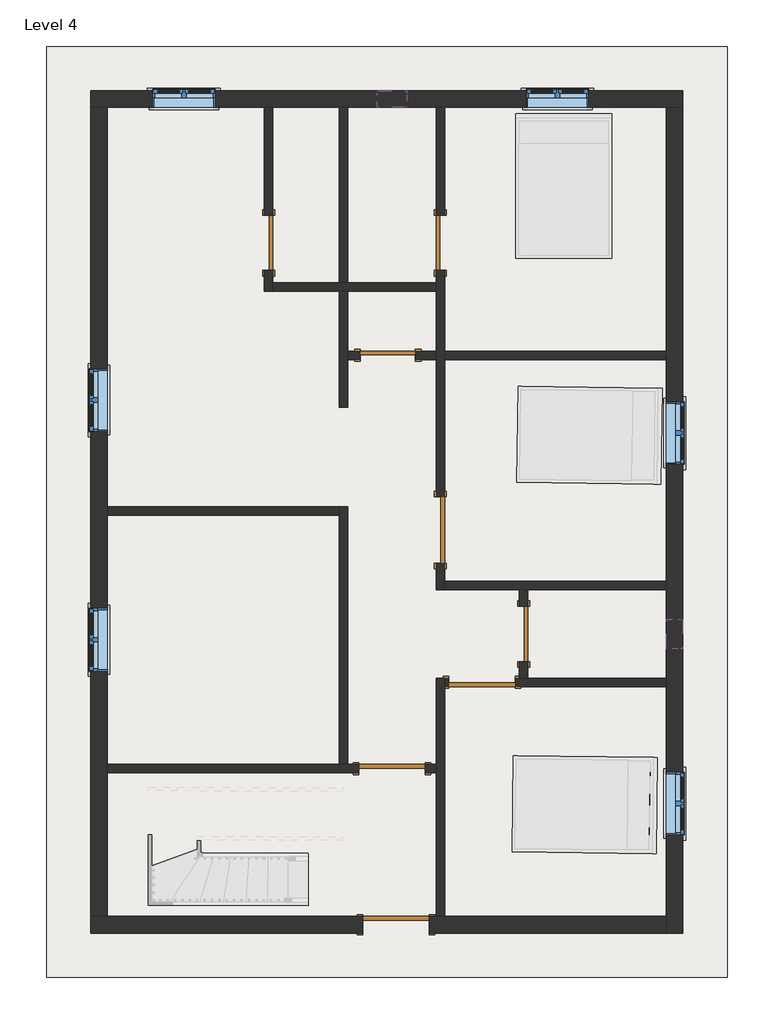
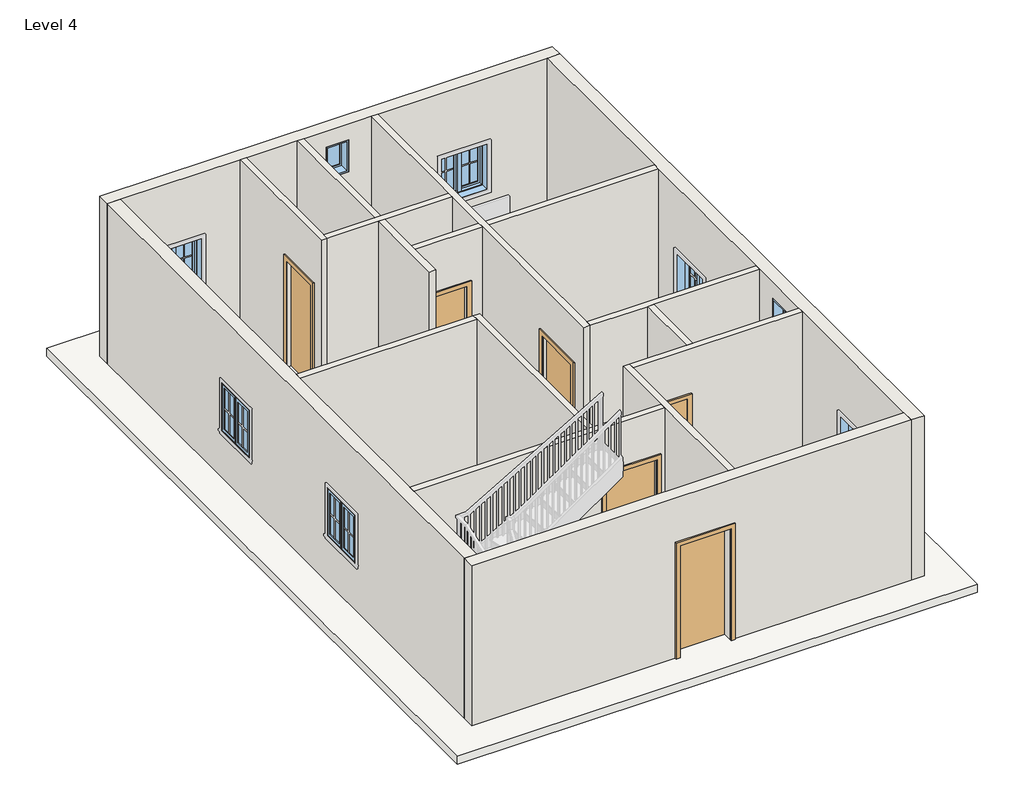
# One storey, part 1 of 3: 17 walls, 8 doors, 8 windows, 1 roof.
"""IFC4 building model written with IfcOpenShell, lengths in millimetres."""

from ifc_helpers import new_model, si_unit, frame, origin, place, context, project, spatial, polyline, outline, extrude, faceted_brep, transform, mapped, element, save
from components import door_d8f5dbb5, door_f2b275c1, door_e5f9f3c4, door_305aa2a5, door_0ca8825f, window_aa618e30, window_339605e1

model = new_model("IFC4")

# Units and contexts
model_context = context("Model", 3, world=origin())
ifc_project = project(units=[si_unit("LENGTHUNIT", "METRE", prefix="MILLI")], contexts=[model_context])

# Site, building, storey
site = spatial("IfcSite", under=ifc_project)
building = spatial("IfcBuilding", under=site)
storey = spatial("IfcBuildingStorey", under=building, Name="Level 4", Elevation=6400.8)

# Doors
placement = place(None, origin())
door_shape = door_d8f5dbb5(model_context)
element("IfcDoor", 1, ObjectType="Single-Flush : 30\" x 80\"", at=placement, inside=storey, context=model_context, shape_type="MappedRepresentation", body=[
    mapped(door_shape, transform((-2883.8867314, 4242.0321212, 6400.8), x_axis=(0.0, -1.0, 0.0), y_axis=(1.0, 0.0, 0.0), z_axis=(0.0, 0.0, 1.0))),
])
door_2_shape = door_f2b275c1(model_context)
element("IfcDoor", 2, ObjectType="Single-Flush : 30\" x 80\"", at=placement, inside=storey, context=model_context, shape_type="MappedRepresentation", body=[
    mapped(door_2_shape, transform((-521.6867314, 4242.0321212, 6400.8), x_axis=(0.0, -1.0, 0.0), y_axis=(1.0, 0.0, 0.0), z_axis=(0.0, 0.0, 1.0))),
])
element("IfcDoor", 3, ObjectType="Single-Flush : 30\" x 80\"", at=placement, inside=storey, context=model_context, shape_type="MappedRepresentation", body=[
    mapped(door_2_shape, transform((-1245.5867314, 2692.6321212, 6400.8), x_axis=(-1.0, 0.0, 0.0), y_axis=(0.0, -1.0, 0.0), z_axis=(0.0, 0.0, 1.0))),
])
element("IfcDoor", 4, ObjectType="Single-Flush : 30\" x 80\"", at=placement, inside=storey, context=model_context, shape_type="MappedRepresentation", body=[
    mapped(door_2_shape, transform((621.3132686, -1136.4178788, 6400.8), x_axis=(0.0, 1.0, 0.0), y_axis=(-1.0, 0.0, 0.0), z_axis=(0.0, 0.0, 1.0))),
])
door_3_shape = door_e5f9f3c4(model_context)
element("IfcDoor", 5, ObjectType="Single-Flush : 36\" x 84\"", at=placement, inside=storey, context=model_context, shape_type="MappedRepresentation", body=[
    mapped(door_3_shape, transform((-521.6867314, 292.3321212, 6400.8), x_axis=(0.0, -1.0, 0.0), y_axis=(1.0, 0.0, 0.0), z_axis=(0.0, 0.0, 1.0))),
])
element("IfcDoor", 6, ObjectType="Single-Flush : 36\" x 84\"", at=placement, inside=storey, context=model_context, shape_type="MappedRepresentation", body=[
    mapped(door_3_shape, transform((-1188.4367314, -2989.1542682, 6400.8), x_axis=(1.0, 0.0, 0.0), y_axis=(0.0, 1.0, 0.0), z_axis=(0.0, 0.0, 1.0))),
])
door_4_shape = door_305aa2a5(model_context)
element("IfcDoor", 7, ObjectType="Single-Flush : 36\" x 84\"", at=placement, inside=storey, context=model_context, shape_type="MappedRepresentation", body=[
    mapped(door_4_shape, transform((49.8132686, -1803.1678788, 6400.8), x_axis=(1.0, 0.0, 0.0), y_axis=(0.0, 1.0, 0.0), z_axis=(0.0, 0.0, 1.0))),
])
door_5_shape = door_0ca8825f(model_context)
element("IfcDoor", 8, ObjectType="Single-Flush : 36\" x 84\"", at=placement, inside=storey, context=model_context, shape_type="MappedRepresentation", body=[
    mapped(door_5_shape, transform((-1131.2867314, -5136.9178788, 6400.8), x_axis=(1.0, 0.0, 0.0), y_axis=(0.0, 1.0, 0.0), z_axis=(0.0, 0.0, 1.0))),
])

# Roof
element("IfcRoof", 9, ObjectType="Generic - 12\"", at=placement, inside=storey, context=model_context, shape_type="SweptSolid", body=[
    extrude(outline(polyline([(-5938.2367314, 6940.7821212), (3421.6632686, 6940.7821212), (3421.6632686, -5860.8178788), (-5938.2367314, -5860.8178788), (-5938.2367314, 6940.7821212)])), frame((0.0, 0.0, 6248.4), z_axis=(0.0, 0.0, 1.0), x_axis=(1.0, 0.0, 0.0)), (0.0, 0.0, 1.0), 152.4),
])

# Walls
element("IfcWall", 10, ObjectType="wall4.5\"", at=placement, inside=storey, context=model_context, shape_type="Brep", body=[
    faceted_brep([(-2941.0367314, 3861.0321212, 8432.8), (-2941.0367314, 3861.0321212, 6400.8), (-2941.0367314, 3575.2821212, 6400.8), (-2941.0367314, 3575.2821212, 9448.8), (-2941.0367314, 6102.5821212, 9448.8), (-2941.0367314, 6102.5821212, 6400.8), (-2941.0367314, 4623.0321212, 6400.8), (-2941.0367314, 4623.0321212, 8432.8), (-2826.7367314, 3575.2821212, 6400.8), (-2826.7367314, 3689.5821212, 6400.8), (-2826.7367314, 3861.0321212, 6400.8), (-2826.7367314, 3861.0321212, 8432.8), (-2826.7367314, 4623.0321212, 8432.8), (-2826.7367314, 4623.0321212, 6400.8), (-2826.7367314, 6102.5821212, 6400.8), (-2826.7367314, 6102.5821212, 9448.8), (-2826.7367314, 3689.5821212, 9448.8), (-2826.7367314, 3575.2821212, 9448.8)], [[[0, 1, 2, 3, 4, 5, 6, 7]], [[8, 9, 10, 11, 12, 13, 14, 15, 16, 17]], [[6, 5, 14, 13]], [[2, 1, 10, 9, 8]], [[5, 4, 15, 14]], [[3, 2, 8, 17]], [[11, 10, 1, 0]], [[12, 11, 0, 7]], [[13, 12, 7, 6]], [[4, 3, 17, 16, 15]]]),
])
element("IfcWall", 11, ObjectType="wall4.5\"", at=placement, inside=storey, context=model_context, shape_type="Brep", body=[
    faceted_brep([(-2826.7367314, 3575.2821212, 6400.8), (-1912.3367314, 3575.2821212, 6400.8), (-1798.0367314, 3575.2821212, 6400.8), (-578.8367314, 3575.2821212, 6400.8), (-578.8367314, 3575.2821212, 9448.8), (-1798.0367314, 3575.2821212, 9448.8), (-1912.3367314, 3575.2821212, 9448.8), (-2826.7367314, 3575.2821212, 9448.8), (-2826.7367314, 3689.5821212, 6400.8), (-2826.7367314, 3689.5821212, 9448.8), (-1912.3367314, 3689.5821212, 9448.8), (-1798.0367314, 3689.5821212, 9448.8), (-578.8367314, 3689.5821212, 9448.8), (-578.8367314, 3689.5821212, 6400.8), (-1798.0367314, 3689.5821212, 6400.8), (-1912.3367314, 3689.5821212, 6400.8)], [[[0, 1, 2, 3, 4, 5, 6, 7]], [[8, 9, 10, 11, 12, 13, 14, 15]], [[3, 2, 1, 0, 8, 15, 14, 13]], [[0, 7, 9, 8]], [[4, 3, 13, 12]], [[7, 6, 5, 4, 12, 11, 10, 9]]]),
])
element("IfcWall", 12, ObjectType="wall4.5\"", at=placement, inside=storey, context=model_context, shape_type="SweptSolid", body=[
    extrude(outline(polyline([(-1912.3367314, 3689.5821212), (-1912.3367314, 6102.5821212), (-1798.0367314, 6102.5821212), (-1798.0367314, 3689.5821212), (-1912.3367314, 3689.5821212)])), frame((0.0, 0.0, 6400.8), z_axis=(0.0, 0.0, 1.0), x_axis=(1.0, 0.0, 0.0)), (0.0, 0.0, 1.0), 3048.0),
])
element("IfcWall", 13, ObjectType="wall4.5\"", at=placement, inside=storey, context=model_context, shape_type="Brep", body=[
    faceted_brep([(-578.8367314, -164.8678788, 8534.4), (-578.8367314, -164.8678788, 6400.8), (-578.8367314, -526.8178788, 6400.8), (-578.8367314, -526.8178788, 9448.8), (-578.8367314, 2635.4821212, 9448.8), (-578.8367314, 2749.7821212, 9448.8), (-578.8367314, 3575.2821212, 9448.8), (-578.8367314, 3689.5821212, 9448.8), (-578.8367314, 6102.5821212, 9448.8), (-578.8367314, 6102.5821212, 6400.8), (-578.8367314, 4623.0321212, 6400.8), (-578.8367314, 4623.0321212, 8432.8), (-578.8367314, 3861.0321212, 8432.8), (-578.8367314, 3861.0321212, 6400.8), (-578.8367314, 3689.5821212, 6400.8), (-578.8367314, 3575.2821212, 6400.8), (-578.8367314, 2749.7821212, 6400.8), (-578.8367314, 2635.4821212, 6400.8), (-578.8367314, 749.5321212, 6400.8), (-578.8367314, 749.5321212, 8534.4), (-464.5367314, -526.8178788, 6400.8), (-464.5367314, -412.5178788, 6400.8), (-464.5367314, -164.8678788, 6400.8), (-464.5367314, -164.8678788, 8534.4), (-464.5367314, 749.5321212, 8534.4), (-464.5367314, 749.5321212, 6400.8), (-464.5367314, 2635.4821212, 6400.8), (-464.5367314, 2749.7821212, 6400.8), (-464.5367314, 3861.0321212, 6400.8), (-464.5367314, 3861.0321212, 8432.8), (-464.5367314, 4623.0321212, 8432.8), (-464.5367314, 4623.0321212, 6400.8), (-464.5367314, 6102.5821212, 6400.8), (-464.5367314, 6102.5821212, 9448.8), (-464.5367314, 2749.7821212, 9448.8), (-464.5367314, 2635.4821212, 9448.8), (-464.5367314, -412.5178788, 9448.8), (-464.5367314, -526.8178788, 9448.8)], [[[0, 1, 2, 3, 4, 5, 6, 7, 8, 9, 10, 11, 12, 13, 14, 15, 16, 17, 18, 19]], [[20, 21, 22, 23, 24, 25, 26, 27, 28, 29, 30, 31, 32, 33, 34, 35, 36, 37]], [[10, 9, 32, 31]], [[2, 1, 22, 21, 20]], [[18, 17, 16, 15, 14, 13, 28, 27, 26, 25]], [[9, 8, 33, 32]], [[3, 2, 20, 37]], [[29, 28, 13, 12]], [[30, 29, 12, 11]], [[31, 30, 11, 10]], [[23, 22, 1, 0]], [[24, 23, 0, 19]], [[25, 24, 19, 18]], [[8, 7, 6, 5, 4, 3, 37, 36, 35, 34, 33]]]),
])
element("IfcWall", 14, ObjectType="wall4.5\"", at=placement, inside=storey, context=model_context, shape_type="Brep", body=[
    faceted_brep([(-464.5367314, -526.8178788, 6400.8), (564.1632686, -526.8178788, 6400.8), (678.4632686, -526.8178788, 6400.8), (2583.4632686, -526.8178788, 6400.8), (2583.4632686, -526.8178788, 9448.8), (678.4632686, -526.8178788, 9448.8), (564.1632686, -526.8178788, 9448.8), (-464.5367314, -526.8178788, 9448.8), (-464.5367314, -412.5178788, 6400.8), (-464.5367314, -412.5178788, 9448.8), (2583.4632686, -412.5178788, 9448.8), (2583.4632686, -412.5178788, 6400.8)], [[[0, 1, 2, 3, 4, 5, 6, 7]], [[8, 9, 10, 11]], [[3, 2, 1, 0, 8, 11]], [[0, 7, 9, 8]], [[4, 3, 11, 10]], [[7, 6, 5, 4, 10, 9]]]),
])
element("IfcWall", 15, ObjectType="wall4.5\"", at=placement, inside=storey, context=model_context, shape_type="SweptSolid", body=[
    extrude(outline(polyline([(2583.4632686, 2749.7821212), (2583.4632686, 2635.4821212), (-464.5367314, 2635.4821212), (-464.5367314, 2749.7821212), (2583.4632686, 2749.7821212)])), frame((0.0, 0.0, 6400.8), z_axis=(0.0, 0.0, 1.0), x_axis=(1.0, 0.0, 0.0)), (0.0, 0.0, 1.0), 3048.0),
    extrude(outline(polyline([(9448.8, -1798.0367314), (6400.8, -1798.0367314), (6400.8, -1626.5867314), (8432.8, -1626.5867314), (8432.8, -864.5867314), (6400.8, -864.5867314), (6400.8, -578.8367314), (9448.8, -578.8367314), (9448.8, -1798.0367314)])), frame((0.0, 2635.4821212, 0.0), z_axis=(0.0, 1.0, 0.0), x_axis=(0.0, 0.0, 1.0)), (0.0, 0.0, 1.0), 114.3),
])
element("IfcWall", 16, ObjectType="wall4.5\"", at=placement, inside=storey, context=model_context, shape_type="Brep", body=[
    faceted_brep([(-1912.3367314, 3575.2821212, 6400.8), (-1912.3367314, 1982.8957318, 6400.8), (-1912.3367314, 1982.8957318, 9448.8), (-1912.3367314, 3575.2821212, 9448.8), (-1798.0367314, 3575.2821212, 6400.8), (-1798.0367314, 3575.2821212, 9448.8), (-1798.0367314, 2749.7821212, 9448.8), (-1798.0367314, 2635.4821212, 9448.8), (-1798.0367314, 1982.8957318, 9448.8), (-1798.0367314, 1982.8957318, 6400.8), (-1798.0367314, 2635.4821212, 6400.8), (-1798.0367314, 2749.7821212, 6400.8)], [[[0, 1, 2, 3]], [[4, 5, 6, 7, 8, 9, 10, 11]], [[1, 0, 4, 11, 10, 9]], [[2, 1, 9, 8]], [[0, 3, 5, 4]], [[3, 2, 8, 7, 6, 5]]]),
])
element("IfcWall", 17, ObjectType="wall4.5\"", at=placement, inside=storey, context=model_context, shape_type="Brep", body=[
    faceted_brep([(-1912.3367314, 611.2957318, 6400.8), (-1912.3367314, 496.9957318, 6400.8), (-1912.3367314, -2932.0042682, 6400.8), (-1912.3367314, -2932.0042682, 9448.8), (-1912.3367314, 496.9957318, 9448.8), (-1912.3367314, 611.2957318, 9448.8), (-1798.0367314, 611.2957318, 6400.8), (-1798.0367314, 611.2957318, 9448.8), (-1798.0367314, -2932.0042682, 9448.8), (-1798.0367314, -2932.0042682, 6400.8)], [[[0, 1, 2, 3, 4, 5]], [[6, 7, 8, 9]], [[2, 1, 0, 6, 9]], [[3, 2, 9, 8]], [[0, 5, 7, 6]], [[5, 4, 3, 8, 7]]]),
])
element("IfcWall", 18, ObjectType="wall4.5\"", at=placement, inside=storey, context=model_context, shape_type="Brep", body=[
    faceted_brep([(-731.2367314, -3046.3042682, 8534.4), (-731.2367314, -3046.3042682, 6400.8), (-578.8367314, -3046.3042682, 6400.8), (-578.8367314, -3046.3042682, 9448.8), (-5100.0367314, -3046.3042682, 9448.8), (-5100.0367314, -3046.3042682, 6400.8), (-1645.6367314, -3046.3042682, 6400.8), (-1645.6367314, -3046.3042682, 8534.4), (-578.8367314, -2932.0042682, 6400.8), (-731.2367314, -2932.0042682, 6400.8), (-731.2367314, -2932.0042682, 8534.4), (-1645.6367314, -2932.0042682, 8534.4), (-1645.6367314, -2932.0042682, 6400.8), (-1798.0367314, -2932.0042682, 6400.8), (-1912.3367314, -2932.0042682, 6400.8), (-5100.0367314, -2932.0042682, 6400.8), (-5100.0367314, -2932.0042682, 9448.8), (-1912.3367314, -2932.0042682, 9448.8), (-1798.0367314, -2932.0042682, 9448.8), (-578.8367314, -2932.0042682, 9448.8)], [[[0, 1, 2, 3, 4, 5, 6, 7]], [[8, 9, 10, 11, 12, 13, 14, 15, 16, 17, 18, 19]], [[6, 5, 15, 14, 13, 12]], [[2, 1, 9, 8]], [[5, 4, 16, 15]], [[3, 2, 8, 19]], [[10, 9, 1, 0]], [[11, 10, 0, 7]], [[12, 11, 7, 6]], [[4, 3, 19, 18, 17, 16]]]),
])
element("IfcWall", 19, ObjectType="wall4.5\"", at=placement, inside=storey, context=model_context, shape_type="Brep", body=[
    faceted_brep([(-464.5367314, -5022.6178788, 6400.8), (-464.5367314, -1860.3178788, 6400.8), (-464.5367314, -1746.0178788, 6400.8), (-464.5367314, -1746.0178788, 9448.8), (-464.5367314, -1860.3178788, 9448.8), (-464.5367314, -5022.6178788, 9448.8), (-578.8367314, -5022.6178788, 6400.8), (-578.8367314, -5022.6178788, 9448.8), (-578.8367314, -3046.3042682, 9448.8), (-578.8367314, -2932.0042682, 9448.8), (-578.8367314, -1746.0178788, 9448.8), (-578.8367314, -1746.0178788, 6400.8), (-578.8367314, -2932.0042682, 6400.8), (-578.8367314, -3046.3042682, 6400.8)], [[[0, 1, 2, 3, 4, 5]], [[6, 7, 8, 9, 10, 11, 12, 13]], [[2, 1, 0, 6, 13, 12, 11]], [[0, 5, 7, 6]], [[3, 2, 11, 10]], [[5, 4, 3, 10, 9, 8, 7]]]),
])
element("IfcWall", 20, ObjectType="wall4.5\"", at=placement, inside=storey, context=model_context, shape_type="Brep", body=[
    faceted_brep([(507.0132686, -1860.3178788, 8534.4), (507.0132686, -1860.3178788, 6400.8), (2583.4632686, -1860.3178788, 6400.8), (2583.4632686, -1860.3178788, 9448.8), (-464.5367314, -1860.3178788, 9448.8), (-464.5367314, -1860.3178788, 6400.8), (-407.3867314, -1860.3178788, 6400.8), (-407.3867314, -1860.3178788, 8534.4), (2583.4632686, -1746.0178788, 6400.8), (678.4632686, -1746.0178788, 6400.8), (564.1632686, -1746.0178788, 6400.8), (507.0132686, -1746.0178788, 6400.8), (507.0132686, -1746.0178788, 8534.4), (-407.3867314, -1746.0178788, 8534.4), (-407.3867314, -1746.0178788, 6400.8), (-464.5367314, -1746.0178788, 6400.8), (-464.5367314, -1746.0178788, 9448.8), (564.1632686, -1746.0178788, 9448.8), (678.4632686, -1746.0178788, 9448.8), (2583.4632686, -1746.0178788, 9448.8)], [[[0, 1, 2, 3, 4, 5, 6, 7]], [[8, 9, 10, 11, 12, 13, 14, 15, 16, 17, 18, 19]], [[6, 5, 15, 14]], [[2, 1, 11, 10, 9, 8]], [[5, 4, 16, 15]], [[3, 2, 8, 19]], [[12, 11, 1, 0]], [[13, 12, 0, 7]], [[14, 13, 7, 6]], [[4, 3, 19, 18, 17, 16]]]),
])
element("IfcWall", 21, ObjectType="wall4.5\"", at=placement, inside=storey, context=model_context, shape_type="SweptSolid", body=[
    extrude(outline(polyline([(-526.8178788, 6400.8), (-755.4178788, 6400.8), (-755.4178788, 8432.8), (-1517.4178788, 8432.8), (-1517.4178788, 6400.8), (-1746.0178788, 6400.8), (-1746.0178788, 9448.8), (-526.8178788, 9448.8), (-526.8178788, 6400.8)])), frame((564.1632686, 0.0, 0.0), z_axis=(1.0, 0.0, 0.0), x_axis=(0.0, 1.0, 0.0)), (0.0, 0.0, 1.0), 114.3),
])
element("IfcWall", 22, ObjectType="wall4.5\"", at=placement, inside=storey, context=model_context, shape_type="SweptSolid", body=[
    extrude(outline(polyline([(-5100.0367314, 611.2957318), (-1912.3367314, 611.2957318), (-1912.3367314, 496.9957318), (-5100.0367314, 496.9957318), (-5100.0367314, 611.2957318)])), frame((0.0, 0.0, 6400.8), z_axis=(0.0, 0.0, 1.0), x_axis=(1.0, 0.0, 0.0)), (0.0, 0.0, 1.0), 3048.0),
])
element("IfcWall", 23, ObjectType="wall9\"", at=placement, inside=storey, context=model_context, shape_type="Brep", body=[
    faceted_brep([(-5328.6367314, 6102.5821212, 6400.8), (-5100.0367314, 6102.5821212, 6400.8), (-2941.0367314, 6102.5821212, 6400.8), (-2826.7367314, 6102.5821212, 6400.8), (-1912.3367314, 6102.5821212, 6400.8), (-1798.0367314, 6102.5821212, 6400.8), (-578.8367314, 6102.5821212, 6400.8), (-464.5367314, 6102.5821212, 6400.8), (2583.4632686, 6102.5821212, 6400.8), (2812.0632686, 6102.5821212, 6400.8), (2812.0632686, 6102.5821212, 9448.8), (2583.4632686, 6102.5821212, 9448.8), (-464.5367314, 6102.5821212, 9448.8), (-578.8367314, 6102.5821212, 9448.8), (-1798.0367314, 6102.5821212, 9448.8), (-1912.3367314, 6102.5821212, 9448.8), (-2826.7367314, 6102.5821212, 9448.8), (-2941.0367314, 6102.5821212, 9448.8), (-5100.0367314, 6102.5821212, 9448.8), (-5328.6367314, 6102.5821212, 9448.8), (-985.2367314, 6102.5821212, 9144.0), (-985.2367314, 6102.5821212, 8534.4), (-1391.6367314, 6102.5821212, 8534.4), (-1391.6367314, 6102.5821212, 9144.0), (1519.8382686, 6102.5821212, 8229.6), (1519.8382686, 6102.5821212, 7315.2), (656.2382686, 6102.5821212, 7315.2), (656.2382686, 6102.5821212, 8229.6), (-3617.3117314, 6102.5821212, 8229.6), (-3617.3117314, 6102.5821212, 7315.2), (-4480.9117314, 6102.5821212, 7315.2), (-4480.9117314, 6102.5821212, 8229.6), (-5328.6367314, 6331.1821212, 6400.8), (-5328.6367314, 6331.1821212, 9448.8), (2812.0632686, 6331.1821212, 9448.8), (2812.0632686, 6331.1821212, 6400.8), (-985.2367314, 6331.1821212, 9144.0), (-1391.6367314, 6331.1821212, 9144.0), (-1391.6367314, 6331.1821212, 8534.4), (-985.2367314, 6331.1821212, 8534.4), (1519.8382686, 6331.1821212, 8229.6), (656.2382686, 6331.1821212, 8229.6), (656.2382686, 6331.1821212, 7315.2), (1519.8382686, 6331.1821212, 7315.2), (-3617.3117314, 6331.1821212, 8229.6), (-4480.9117314, 6331.1821212, 8229.6), (-4480.9117314, 6331.1821212, 7315.2), (-3617.3117314, 6331.1821212, 7315.2)], [[[0, 1, 2, 3, 4, 5, 6, 7, 8, 9, 10, 11, 12, 13, 14, 15, 16, 17, 18, 19], [20, 21, 22, 23], [24, 25, 26, 27], [28, 29, 30, 31]], [[32, 33, 34, 35], [36, 37, 38, 39], [40, 41, 42, 43], [44, 45, 46, 47]], [[9, 8, 7, 6, 5, 4, 3, 2, 1, 0, 32, 35]], [[10, 9, 35, 34]], [[0, 19, 33, 32]], [[21, 20, 36, 39]], [[22, 21, 39, 38]], [[23, 22, 38, 37]], [[20, 23, 37, 36]], [[25, 24, 40, 43]], [[26, 25, 43, 42]], [[27, 26, 42, 41]], [[24, 27, 41, 40]], [[29, 28, 44, 47]], [[30, 29, 47, 46]], [[31, 30, 46, 45]], [[28, 31, 45, 44]], [[19, 18, 17, 16, 15, 14, 13, 12, 11, 10, 34, 33]]]),
])
element("IfcWall", 24, ObjectType="wall9\"", at=placement, inside=storey, context=model_context, shape_type="Brep", body=[
    faceted_brep([(2583.4632686, 6102.5821212, 6400.8), (2583.4632686, 2749.7821212, 6400.8), (2583.4632686, 2635.4821212, 6400.8), (2583.4632686, -412.5178788, 6400.8), (2583.4632686, -526.8178788, 6400.8), (2583.4632686, -1746.0178788, 6400.8), (2583.4632686, -1860.3178788, 6400.8), (2583.4632686, -5022.6178788, 6400.8), (2583.4632686, -5251.2178788, 6400.8), (2583.4632686, -5251.2178788, 9448.8), (2583.4632686, -5022.6178788, 9448.8), (2583.4632686, -1860.3178788, 9448.8), (2583.4632686, -1746.0178788, 9448.8), (2583.4632686, -526.8178788, 9448.8), (2583.4632686, -412.5178788, 9448.8), (2583.4632686, 2635.4821212, 9448.8), (2583.4632686, 2749.7821212, 9448.8), (2583.4632686, 6102.5821212, 9448.8), (2583.4632686, -1339.6178788, 9144.0), (2583.4632686, -1339.6178788, 8534.4), (2583.4632686, -933.2178788, 8534.4), (2583.4632686, -933.2178788, 9144.0), (2583.4632686, 1194.0321212, 8229.6), (2583.4632686, 1194.0321212, 7315.2), (2583.4632686, 2057.6321212, 7315.2), (2583.4632686, 2057.6321212, 8229.6), (2583.4632686, -3901.8428788, 8229.6), (2583.4632686, -3901.8428788, 7315.2), (2583.4632686, -3038.2428788, 7315.2), (2583.4632686, -3038.2428788, 8229.6), (2812.0632686, 6102.5821212, 6400.8), (2812.0632686, 6102.5821212, 9448.8), (2812.0632686, -5251.2178788, 9448.8), (2812.0632686, -5251.2178788, 6400.8), (2812.0632686, -1339.6178788, 9144.0), (2812.0632686, -933.2178788, 9144.0), (2812.0632686, -933.2178788, 8534.4), (2812.0632686, -1339.6178788, 8534.4), (2812.0632686, 1194.0321212, 8229.6), (2812.0632686, 2057.6321212, 8229.6), (2812.0632686, 2057.6321212, 7315.2), (2812.0632686, 1194.0321212, 7315.2), (2812.0632686, -3901.8428788, 8229.6), (2812.0632686, -3038.2428788, 8229.6), (2812.0632686, -3038.2428788, 7315.2), (2812.0632686, -3901.8428788, 7315.2)], [[[0, 1, 2, 3, 4, 5, 6, 7, 8, 9, 10, 11, 12, 13, 14, 15, 16, 17], [18, 19, 20, 21], [22, 23, 24, 25], [26, 27, 28, 29]], [[30, 31, 32, 33], [34, 35, 36, 37], [38, 39, 40, 41], [42, 43, 44, 45]], [[8, 7, 6, 5, 4, 3, 2, 1, 0, 30, 33]], [[0, 17, 31, 30]], [[9, 8, 33, 32]], [[19, 18, 34, 37]], [[20, 19, 37, 36]], [[21, 20, 36, 35]], [[18, 21, 35, 34]], [[23, 22, 38, 41]], [[24, 23, 41, 40]], [[25, 24, 40, 39]], [[22, 25, 39, 38]], [[27, 26, 42, 45]], [[28, 27, 45, 44]], [[29, 28, 44, 43]], [[26, 29, 43, 42]], [[17, 16, 15, 14, 13, 12, 11, 10, 9, 32, 31]]]),
])
element("IfcWall", 25, ObjectType="wall9\"", at=placement, inside=storey, context=model_context, shape_type="Brep", body=[
    faceted_brep([(2583.4632686, -5022.6178788, 6400.8), (-464.5367314, -5022.6178788, 6400.8), (-578.8367314, -5022.6178788, 6400.8), (-674.0867314, -5022.6178788, 6400.8), (-674.0867314, -5022.6178788, 8534.4), (-1588.4867314, -5022.6178788, 8534.4), (-1588.4867314, -5022.6178788, 6400.8), (-5100.0367314, -5022.6178788, 6400.8), (-5328.6367314, -5022.6178788, 6400.8), (-5328.6367314, -5022.6178788, 9448.8), (-5100.0367314, -5022.6178788, 9448.8), (-578.8367314, -5022.6178788, 9448.8), (-464.5367314, -5022.6178788, 9448.8), (2583.4632686, -5022.6178788, 9448.8), (-674.0867314, -5251.2178788, 8534.4), (-674.0867314, -5251.2178788, 6400.8), (2583.4632686, -5251.2178788, 6400.8), (2583.4632686, -5251.2178788, 9448.8), (-5328.6367314, -5251.2178788, 9448.8), (-5328.6367314, -5251.2178788, 6400.8), (-1588.4867314, -5251.2178788, 6400.8), (-1588.4867314, -5251.2178788, 8534.4)], [[[0, 1, 2, 3, 4, 5, 6, 7, 8, 9, 10, 11, 12, 13]], [[14, 15, 16, 17, 18, 19, 20, 21]], [[20, 19, 8, 7, 6]], [[16, 15, 3, 2, 1, 0]], [[0, 13, 17, 16]], [[9, 8, 19, 18]], [[4, 3, 15, 14]], [[5, 4, 14, 21]], [[6, 5, 21, 20]], [[13, 12, 11, 10, 9, 18, 17]]]),
])
element("IfcWall", 26, ObjectType="wall9\"", at=placement, inside=storey, context=model_context, shape_type="Brep", body=[
    faceted_brep([(-5328.6367314, 6102.5821212, 6400.8), (-5328.6367314, -5022.6178788, 6400.8), (-5328.6367314, -5022.6178788, 9448.8), (-5328.6367314, 6102.5821212, 9448.8), (-5328.6367314, 2509.9457318, 8229.6), (-5328.6367314, 1646.3457318, 8229.6), (-5328.6367314, 1646.3457318, 7315.2), (-5328.6367314, 2509.9457318, 7315.2), (-5328.6367314, -785.7042682, 8229.6), (-5328.6367314, -1649.3042682, 8229.6), (-5328.6367314, -1649.3042682, 7315.2), (-5328.6367314, -785.7042682, 7315.2), (-5100.0367314, 6102.5821212, 6400.8), (-5100.0367314, 6102.5821212, 9448.8), (-5100.0367314, 611.2957318, 9448.8), (-5100.0367314, 496.9957318, 9448.8), (-5100.0367314, -2932.0042682, 9448.8), (-5100.0367314, -3046.3042682, 9448.8), (-5100.0367314, -5022.6178788, 9448.8), (-5100.0367314, -5022.6178788, 6400.8), (-5100.0367314, -3046.3042682, 6400.8), (-5100.0367314, -2932.0042682, 6400.8), (-5100.0367314, 496.9957318, 6400.8), (-5100.0367314, 611.2957318, 6400.8), (-5100.0367314, 2509.9457318, 8229.6), (-5100.0367314, 2509.9457318, 7315.2), (-5100.0367314, 1646.3457318, 7315.2), (-5100.0367314, 1646.3457318, 8229.6), (-5100.0367314, -785.7042682, 8229.6), (-5100.0367314, -785.7042682, 7315.2), (-5100.0367314, -1649.3042682, 7315.2), (-5100.0367314, -1649.3042682, 8229.6)], [[[0, 1, 2, 3], [4, 5, 6, 7], [8, 9, 10, 11]], [[12, 13, 14, 15, 16, 17, 18, 19, 20, 21, 22, 23], [24, 25, 26, 27], [28, 29, 30, 31]], [[1, 0, 12, 23, 22, 21, 20, 19]], [[0, 3, 13, 12]], [[2, 1, 19, 18]], [[25, 24, 4, 7]], [[26, 25, 7, 6]], [[27, 26, 6, 5]], [[24, 27, 5, 4]], [[29, 28, 8, 11]], [[30, 29, 11, 10]], [[31, 30, 10, 9]], [[28, 31, 9, 8]], [[3, 2, 18, 17, 16, 15, 14, 13]]]),
])

# Windows
window_shape = window_aa618e30(model_context)
element("IfcWindow", 27, ObjectType="Fixed : 16\" x 24\"", at=placement, inside=storey, context=model_context, shape_type="MappedRepresentation", body=[
    mapped(window_shape, transform((-1150.3367314, 6216.8821212, 7620.0), x_axis=(1.0, 0.0, 0.0), y_axis=(0.0, 1.0, 0.0), z_axis=(0.0, 0.0, 1.0))),
])
element("IfcWindow", 28, ObjectType="Fixed : 16\" x 24\"", at=placement, inside=storey, context=model_context, shape_type="MappedRepresentation", body=[
    mapped(window_shape, transform((2697.7632686, -1174.5178788, 7620.0), x_axis=(0.0, -1.0, 0.0), y_axis=(1.0, 0.0, 0.0), z_axis=(0.0, 0.0, 1.0))),
])
window_2_shape = window_339605e1(model_context)
element("IfcWindow", 29, ObjectType="Window-Casement-Double : 34\" x 36\"", at=placement, inside=storey, context=model_context, shape_type="MappedRepresentation", body=[
    mapped(window_2_shape, transform((1088.0382686, 6216.8821212, 6400.8), x_axis=(1.0, 0.0, 0.0), y_axis=(0.0, 1.0, 0.0), z_axis=(0.0, 0.0, 1.0))),
])
element("IfcWindow", 30, ObjectType="Window-Casement-Double : 34\" x 36\"", at=placement, inside=storey, context=model_context, shape_type="MappedRepresentation", body=[
    mapped(window_2_shape, transform((2697.7632686, 1625.8321212, 6400.8), x_axis=(0.0, -1.0, 0.0), y_axis=(1.0, 0.0, 0.0), z_axis=(0.0, 0.0, 1.0))),
])
element("IfcWindow", 31, ObjectType="Window-Casement-Double : 34\" x 36\"", at=placement, inside=storey, context=model_context, shape_type="MappedRepresentation", body=[
    mapped(window_2_shape, transform((2697.7632686, -3470.0428788, 6400.8), x_axis=(0.0, -1.0, 0.0), y_axis=(1.0, 0.0, 0.0), z_axis=(0.0, 0.0, 1.0))),
])
element("IfcWindow", 32, ObjectType="Window-Casement-Double : 34\" x 36\"", at=placement, inside=storey, context=model_context, shape_type="MappedRepresentation", body=[
    mapped(window_2_shape, transform((-4049.1117314, 6216.8821212, 6400.8), x_axis=(1.0, 0.0, 0.0), y_axis=(0.0, 1.0, 0.0), z_axis=(0.0, 0.0, 1.0))),
])
element("IfcWindow", 33, ObjectType="Window-Casement-Double : 34\" x 36\"", at=placement, inside=storey, context=model_context, shape_type="MappedRepresentation", body=[
    mapped(window_2_shape, transform((-5214.3367314, 2078.1457318, 6400.8), x_axis=(0.0, 1.0, 0.0), y_axis=(-1.0, 0.0, 0.0), z_axis=(0.0, 0.0, 1.0))),
])
element("IfcWindow", 34, ObjectType="Window-Casement-Double : 34\" x 36\"", at=placement, inside=storey, context=model_context, shape_type="MappedRepresentation", body=[
    mapped(window_2_shape, transform((-5214.3367314, -1217.5042682, 6400.8), x_axis=(0.0, 1.0, 0.0), y_axis=(-1.0, 0.0, 0.0), z_axis=(0.0, 0.0, 1.0))),
])

save(model, "model.ifc")

# Revit data of these elements
# Type "Single-Flush : 30\" x 80\""
#   Type Mark = "5"
#   Construction Type Id = "MDOOR"
#   Assembly Code = "C1020"
#   Analytic Construction = "Metal"
#   Thickness = 0' - 2"
#   Heat Transfer Coefficient (U) = 0.651978 BTU/(h·ft²·°F)
#   Height = 6' - 8"
#   Trim Projection Ext = 0' - 1"
#   Trim Projection Int = 0' - 1"
#   Trim Width = 0' - 3"
#   Width = 2' - 6"
#   Define Thermal Properties by = 1
#   Define Thermal Properties by = 1
#   Door Material = Door - Panel
#   Frame Material = Door - Frame
#   Visual Light Transmittance = 0
#   Solar Heat Gain Coefficient = 0
#   Function = (empty or 0)
#   Wall Closure = (empty or 0)
# Type "Single-Flush : 36\" x 84\""
#   Type Mark = "1"
#   Construction Type Id = "MDOOR"
#   Assembly Code = "C1020"
#   Analytic Construction = "Metal"
#   Thickness = 0' - 2"
#   Heat Transfer Coefficient (U) = 0.651978 BTU/(h·ft²·°F)
#   Height = 7' - 0"
#   Trim Projection Ext = 0' - 1"
#   Trim Projection Int = 0' - 1"
#   Trim Width = 0' - 3"
#   Width = 3' - 0"
#   Define Thermal Properties by = 1
#   Define Thermal Properties by = 1
#   Door Material = Door - Panel
#   Frame Material = Door - Frame
#   Visual Light Transmittance = 0
#   Solar Heat Gain Coefficient = 0
#   Function = (empty or 0)
#   Wall Closure = (empty or 0)
# Type "Generic - 12\""
#   Assembly Code = "B1020"
#   Layers, outside or top first: 0' - 6" no material (function 1)
# Type "wall4.5\""
#   Assembly Code = "B2010"
#   Layers, outside or top first: 0' - 4 1/2" no material (function 1)
# Type "wall9\""
#   Assembly Code = "B2010"
#   Layers, outside or top first: 0' - 9" no material (function 1)
# Type "Fixed : 16\" x 24\""
#   Type Mark = "4"
#   Construction Type Id = "GSP4R"
#   Assembly Code = "B2020100"
#   Analytic Construction = "1/8 in Pilkington single glazing"
#   Visual Light Transmittance = 0.9
#   Solar Heat Gain Coefficient = 0.78
#   Heat Transfer Coefficient (U) = 0.6496 BTU/(h·ft²·°F)
#   Height = 2' - 0"
#   Default Sill Height = 3' - 0"
#   Width = 1' - 4"
#   Window Inset = 0' - 0 3/4"
#   Define Thermal Properties by = 1
#   Define Thermal Properties by = 1
#   Glass Pane Material = Glass
#   Sash Material = Sash
#   Wall Closure = (empty or 0)
# Type "Window-Casement-Double : 34\" x 36\""
#   Type Mark = "14"
#   Fire Rating = "0.5h"
#   Assembly Code = "B2020100"
#   Analytic Construction = "Double glazing - domestic"
#   Frame Extension [instance default] = 0' - 0 1/4"
#   Window Inset [instance default] = 0' - 0"
#   Wall Thickness [instance default] = 0' - 6"
#   Interior Wall Closure [instance default] = 0' - 2 1/4"
#   Half Width = 1' - 5"
#   Visual Light Transmittance = 0.81
#   Thermal Resistance (R) = 1.8146 (h·ft²·°F)/BTU
#   Solar Heat Gain Coefficient = 0.76
#   Rough Width = 2' - 10 1/2"
#   Rough Height = 3' - 0 1/2"
#   Height = 3' - 0"
#   Heat Transfer Coefficient (U) = 0.5511 BTU/(h·ft²·°F)
#   Exterior Wall Closure [instance default] = 0' - 1 1/4"
#   Extension Jamb [instance default] = 0' - 2 1/4"
#   Default Sill Height = 3' - 0"
#   Width = 2' - 10"
#   Define Thermal Properties by = 0
#   Muntin Visibility = yes
#   Interior Trim Visibility [instance default] = yes
#   Exterior Trim Visibility [instance default] = yes
#   Extension Jamb Visibility [instance default] = yes
#   Interior Trim Material = Wood - Stained
#   Muntin Pattern = Muntin Pattern_2x2 : Muntin Pattern_2x2
#   Interior Trim = Trim-Window-Interior-Flat : Picture Frame
#   Interior Frame Material = Wood - Stained
#   Glass Panel Material = Glass
#   Exterior Trim Material = Clad - White
#   Exterior Trim = Trim-Window-Exterior-Flat : with Sill
#   Exterior Frame Material = Clad - White
#   Wall Closure = (empty or 0)
# Elements 1, 2, 3, 4 (IfcDoor, "Single-Flush : 30\" x 80\"")
#   Phase Created = New Construction
#   Materials on its faces: "Door - Frame", "Door - Panel"
# Elements 5, 6, 7, 8 (IfcDoor, "Single-Flush : 36\" x 84\"")
#   Phase Created = New Construction
#   Materials on its faces: "Door - Frame", "Door - Panel"
# Element 9 (IfcRoof, "Generic - 12\"")
#   built-in parameter 1001705 = 21 (stored number, unit not read)
#   built-in parameter 1001701 = -0.5 (stored number, unit not read)
#   built-in parameter 1001710 = 33615
#   Phase Created = New Construction
#   Materials on its faces: "Default Roof"
# Elements 10, 11, 12, 13, 14, 15, 16, 17, 18, 19, 20, 21, 22 (IfcWall, "wall4.5\"")
#   Top Offset = 0' - 0"
#   Base Offset = 0' - 0"
#   Unconnected Height = 10' - 0"
#   wall height = 10' - 0"
#   Phase Created = New Construction
#   Base Constraint = Level 4
#   Materials on its faces: "Default Wall"
# Elements 23, 24, 25, 26 (IfcWall, "wall9\"")
#   Top Offset = 0' - 0"
#   Base Offset = 0' - 0"
#   Unconnected Height = 10' - 0"
#   wall height = 10' - 0"
#   Phase Created = New Construction
#   Base Constraint = Level 4
#   Materials on its faces: "Default Wall", "Wood Planks"
# Element 27 (IfcWindow, "Fixed : 16\" x 24\"")
#   Mark = "17"
#   Phase Created = New Construction
#   Materials on its faces: "Sash", "Glass"
# Element 28 (IfcWindow, "Fixed : 16\" x 24\"")
#   Mark = "18"
#   Phase Created = New Construction
#   Materials on its faces: "Sash", "Glass"
# Element 29 (IfcWindow, "Window-Casement-Double : 34\" x 36\"")
#   Mark = "19"
#   Window Inset = 0' - 0"
#   Interior Wall Closure = 0' - 2 1/4"
#   Frame Extension = 0' - 0 1/4"
#   Exterior Wall Closure = 0' - 1 1/4"
#   Interior Trim Visibility = yes
#   Exterior Trim Visibility = yes
#   Phase Created = New Construction
#   Materials on its faces: "Wood - Stained", "Glass", "Clad - White"
# Element 30 (IfcWindow, "Window-Casement-Double : 34\" x 36\"")
#   Mark = "20"
#   Window Inset = 0' - 0"
#   Interior Wall Closure = 0' - 2 1/4"
#   Frame Extension = 0' - 0 1/4"
#   Exterior Wall Closure = 0' - 1 1/4"
#   Interior Trim Visibility = yes
#   Exterior Trim Visibility = yes
#   Phase Created = New Construction
#   Materials on its faces: "Wood - Stained", "Glass", "Clad - White"
# Element 31 (IfcWindow, "Window-Casement-Double : 34\" x 36\"")
#   Mark = "21"
#   Window Inset = 0' - 0"
#   Interior Wall Closure = 0' - 2 1/4"
#   Frame Extension = 0' - 0 1/4"
#   Exterior Wall Closure = 0' - 1 1/4"
#   Interior Trim Visibility = yes
#   Exterior Trim Visibility = yes
#   Phase Created = New Construction
#   Materials on its faces: "Wood - Stained", "Glass", "Clad - White"
# Element 32 (IfcWindow, "Window-Casement-Double : 34\" x 36\"")
#   Mark = "22"
#   Window Inset = 0' - 0"
#   Interior Wall Closure = 0' - 2 1/4"
#   Frame Extension = 0' - 0 1/4"
#   Exterior Wall Closure = 0' - 1 1/4"
#   Interior Trim Visibility = yes
#   Exterior Trim Visibility = yes
#   Phase Created = New Construction
#   Materials on its faces: "Wood - Stained", "Glass", "Clad - White"
# Element 33 (IfcWindow, "Window-Casement-Double : 34\" x 36\"")
#   Mark = "23"
#   Window Inset = 0' - 0"
#   Interior Wall Closure = 0' - 2 1/4"
#   Frame Extension = 0' - 0 1/4"
#   Exterior Wall Closure = 0' - 1 1/4"
#   Interior Trim Visibility = yes
#   Exterior Trim Visibility = yes
#   Phase Created = New Construction
#   Materials on its faces: "Wood - Stained", "Glass", "Clad - White"
# Element 34 (IfcWindow, "Window-Casement-Double : 34\" x 36\"")
#   Mark = "24"
#   Window Inset = 0' - 0"
#   Interior Wall Closure = 0' - 2 1/4"
#   Frame Extension = 0' - 0 1/4"
#   Exterior Wall Closure = 0' - 1 1/4"
#   Interior Trim Visibility = yes
#   Exterior Trim Visibility = yes
#   Phase Created = New Construction
#   Materials on its faces: "Wood - Stained", "Glass", "Clad - White"
# Materials
#   "Door - Panel": class "Wood", colour RGB 210 159 95, transparency 0, Cost = 0
#   "Door - Frame": colour RGB 118 70 51, transparency 0, Cost = 0
#   "Glass": class "Glass", colour RGB 0 128 192, transparency 0.75, Description = "Soda Lime Glass", Cost = 0
#   "Sash": class "Wood", colour RGB 224 178 126, transparency 0, Cost = 0
#   "Wood - Stained": class "Wood", colour RGB 224 178 126, transparency 0, Cost = 0
#   "Clad - White": class "Wood", colour RGB 242 242 238, transparency 0, Cost = 0
#   "Default Roof": colour RGB 88 101 114, transparency 0, Cost = 0
#   "Default Wall": colour RGB 128 128 128, transparency 0, Cost = 0
#   "Wood Planks": class "Wood", colour RGB 193 160 115, transparency 0, Description = "Physical material.", Cost = 0
